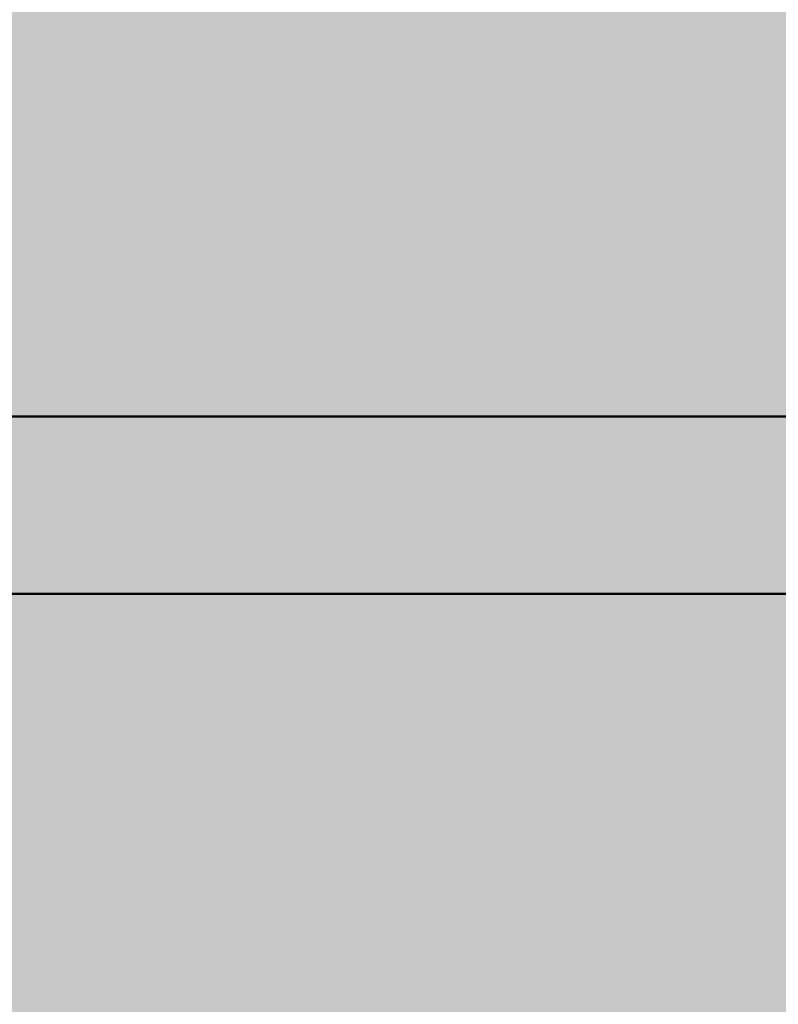
# Model space of a CAD drawing. Units: millimetres. Extents: x 0 to 2267, y 0 to 1823.
# Tile 132 of 256: x 1611 to 1632, y 1216 to 1243. Entities that reach past the tile are written whole.
import ezdxf

# ---------------------------------------------------------------- set-up
doc = ezdxf.new("R2010")
doc.units = ezdxf.units.MM
doc.header["$MEASUREMENT"] = 0
doc.layers.add('M-HATC', color=252, linetype='Continuous', lineweight=18)
doc.layers.add('M-OUTL', color=7, linetype='Continuous', lineweight=50)

msp = doc.modelspace()

# ---------------------------------------------------------------- hatches: boundary and pattern name
at = {"layer": 'M-HATC'}
h = msp.add_hatch(color=256, dxfattribs=at)
h.dxf.hatch_style = 1
h.paths.add_polyline_path([(2065.771, 1618.062, 0.236068), (2055.771, 1638.062), (1381.087, 1638.062, 0.236068), (1371.087, 1618.062), (1371.087, 1603.062), (2055.771, 1603.062), (2065.771, 1603.062)])
h.paths.add_polyline_path([(2062.772, 1550.296), (2062.772, 1560.296), (1374.086, 1560.296), (1374.086, 1550.296), (1374.086, 1540.296), (1384.086, 1540.296), (1389.086, 1540.296), (2062.772, 1540.296)])
h.paths.add_polyline_path([(1930.929, 1282.766), (1505.929, 1282.766), (1587.628, 1235.597, 0.131652), (1600.128, 1232.247), (1836.73, 1232.247, 0.131652), (1849.23, 1235.597)])
h.paths.add_polyline_path([(1930.929, 1117.417), (1905.929, 1117.417), (1505.929, 1117.417), (1505.929, 1077.417), (1930.929, 1077.417)])
h = msp.add_hatch(color=256, dxfattribs=at)
h.dxf.hatch_style = 1
h.paths.add_polyline_path([(2055.771, 1603.062), (1381.087, 1603.062), (1381.087, 1598.062), (2055.771, 1598.062)])
h.paths.add_polyline_path([(2055.771, 1598.062), (1381.087, 1598.062), (1381.087, 1593.062), (2055.771, 1593.062)])
h.paths.add_polyline_path([(2051.307, 1536.761), (1385.55, 1536.761), (1385.55, 1526.761), (1387.55, 1526.761), (1388.537, 1525.053), (1385.332, 1521.233), (1385.332, 1521.223), (2050.254, 1522.749), (2048.321, 1525.053), (2049.307, 1526.761), (2051.307, 1526.761)])
edge = h.paths.add_edge_path()
edge.add_arc((1847.535, 1379.149), 135, 222.60306, 222.89085, ccw=False)
edge.add_line((1748.166, 1287.766), (1683.092, 1287.766))
edge.add_arc((1583.724, 1379.149), 135, 317.10915, 317.39694, ccw=False)
edge.add_arc((1678.969, 1290.671), 5, 222.8909, 317.1091, ccw=False)
edge.add_arc((1774.213, 1379.149), 135, 222.60306, 222.89085, ccw=False)
edge.add_line((1674.845, 1287.766), (1609.771, 1287.766))
edge.add_arc((1510.403, 1379.149), 135, 317.10915, 317.39694, ccw=False)
edge.add_arc((1605.647, 1290.671), 5, 222.8909, 317.1091, ccw=False)
edge.add_arc((1700.892, 1379.149), 135, 222.60306, 222.89085, ccw=False)
edge.add_line((1601.524, 1287.766), (1536.45, 1287.766))
edge.add_arc((1437.081, 1379.149), 135, 317.10915, 317.39694, ccw=False)
edge.add_arc((1532.326, 1290.671), 5, 222.8909, 317.1091, ccw=False)
edge.add_arc((1627.571, 1379.149), 135, 222.60306, 222.89085, ccw=False)
edge.add_line((1528.203, 1287.766), (1505.929, 1287.766))
edge.add_spline(control_points=[(1505.929, 1287.766), (1504.262, 1287.766), (1504.262, 1282.766), (1505.929, 1282.766)], knot_values=[0, 0, 0, 0, 5, 5, 5, 5], degree=3, periodic=0)
edge.add_line((1505.929, 1282.766), (1930.929, 1282.766))
edge.add_spline(control_points=[(1930.929, 1282.766), (1932.596, 1282.766), (1932.596, 1287.766), (1930.929, 1287.766)], knot_values=[0, 0, 0, 0, 5, 5, 5, 5], degree=3, periodic=0)
edge.add_line((1930.929, 1287.766), (1903.056, 1287.766))
edge.add_arc((1803.688, 1379.149), 135, 317.10915, 317.39694, ccw=False)
edge.add_arc((1898.932, 1290.671), 5, 222.8909, 317.1091, ccw=False)
edge.add_arc((1994.177, 1379.149), 135, 222.60306, 222.89085, ccw=False)
edge.add_line((1894.809, 1287.766), (1829.735, 1287.766))
edge.add_arc((1730.366, 1379.149), 135, 317.10915, 317.39694, ccw=False)
edge.add_arc((1825.611, 1290.671), 5, 222.8909, 317.1091, ccw=False)
edge.add_arc((1920.856, 1379.149), 135, 222.60306, 222.89085, ccw=False)
edge.add_line((1821.487, 1287.766), (1756.413, 1287.766))
edge.add_arc((1657.045, 1379.149), 135, 317.10915, 317.39694, ccw=False)
edge.add_arc((1752.29, 1290.671), 5, 222.8909, 317.1091, ccw=False)
edge = h.paths.add_edge_path()
edge.add_spline(control_points=[(1843.429, 1227.247), (1845.096, 1227.247), (1845.096, 1232.247), (1843.429, 1232.247)], knot_values=[0, 0, 0, 0, 5, 5, 5, 5], degree=3, periodic=0)
edge.add_line((1843.429, 1232.247), (1593.429, 1232.247))
edge.add_spline(control_points=[(1593.429, 1232.247), (1591.762, 1232.247), (1591.762, 1227.247), (1593.429, 1227.247)], knot_values=[0, 0, 0, 0, 5, 5, 5, 5], degree=3, periodic=0)
edge.add_line((1593.429, 1227.247), (1843.429, 1227.247))
h.paths.add_polyline_path([(1905.929, 1127.417), (1530.929, 1127.417, 0.414214), (1520.929, 1117.417), (1530.929, 1117.417), (1915.929, 1117.417, 0.414214)])
edge = h.paths.add_edge_path()
edge.add_arc((1397.086, 1498.408), 12.73, 90.7821, 190.8787, ccw=False)
edge.add_line((1396.912, 1511.136), (1428.01, 1511.349))
edge.add_line((1428.01, 1511.349), (1433.01, 1511.349))
edge.add_line((1433.01, 1511.349), (1434.439, 1511.349))
edge.add_arc((1419.474, 1498.08), 20, 41.561, 74.0821)
edge.add_line((1424.959, 1517.314), (1399.935, 1517.256))
edge.add_spline(control_points=[(1399.931, 1517.256), (1399.884, 1517.213), (1399.833, 1517.169), (1399.777, 1517.124)], knot_values=[11.567499, 11.567499, 11.567499, 11.567499, 11.814249, 11.814249, 11.814249, 11.814249], degree=3, periodic=0)
edge.add_spline(control_points=[(1399.633, 1517.01), (1399.583, 1516.972), (1399.531, 1516.934), (1399.476, 1516.895)], knot_values=[11.167718, 11.167718, 11.167718, 11.167718, 11.365188, 11.365188, 11.365188, 11.365188], degree=3, periodic=0)
edge.add_spline(control_points=[(1399.34, 1516.8), (1399.151, 1516.672), (1398.938, 1516.538), (1398.704, 1516.399)], knot_values=[10.376405, 10.376405, 10.376405, 10.376405, 11.00994, 11.00994, 11.00994, 11.00994], degree=3, periodic=0)
edge.add_spline(control_points=[(1398.657, 1516.372), (1398.579, 1516.326), (1398.498, 1516.28), (1398.415, 1516.233)], knot_values=[10.125175, 10.125175, 10.125175, 10.125175, 10.334406, 10.334406, 10.334406, 10.334406], degree=3, periodic=0)
edge.add_spline(control_points=[(1398.264, 1516.149), (1398.196, 1516.111), (1398.126, 1516.073), (1398.055, 1516.035)], knot_values=[9.832246, 9.832246, 9.832246, 9.832246, 9.999658, 9.999658, 9.999658, 9.999658], degree=3, periodic=0)
edge.add_spline(control_points=[(1397.999, 1516.005), (1397.731, 1515.862), (1397.446, 1515.717), (1397.147, 1515.571)], knot_values=[9.161808, 9.161808, 9.161808, 9.161808, 9.787769, 9.787769, 9.787769, 9.787769], degree=3, periodic=0)
edge.add_spline(control_points=[(1397.147, 1515.571), (1396.842, 1515.423), (1396.522, 1515.274), (1396.191, 1515.126)], knot_values=[8.524455, 8.524455, 8.524455, 8.524455, 9.161808, 9.161808, 9.161808, 9.161808], degree=3, periodic=0)
edge.add_spline(control_points=[(1396.078, 1515.076), (1395.985, 1515.035), (1395.892, 1514.994), (1395.798, 1514.953)], knot_values=[8.275193, 8.275193, 8.275193, 8.275193, 8.451726, 8.451726, 8.451726, 8.451726], degree=3, periodic=0)
edge.add_spline(control_points=[(1395.602, 1514.869), (1395.5, 1514.826), (1395.397, 1514.782), (1395.293, 1514.739)], knot_values=[7.962917, 7.962917, 7.962917, 7.962917, 8.152764, 8.152764, 8.152764, 8.152764], degree=3, periodic=0)
edge.add_spline(control_points=[(1395.212, 1514.706), (1394.828, 1514.547), (1394.435, 1514.393), (1394.036, 1514.244)], knot_values=[7.21254, 7.21254, 7.21254, 7.21254, 7.913148, 7.913148, 7.913148, 7.913148], degree=3, periodic=0)
edge.add_spline(control_points=[(1394.036, 1514.244), (1393.708, 1514.121), (1393.375, 1514.003), (1393.043, 1513.889)], knot_values=[6.633733, 6.633733, 6.633733, 6.633733, 7.21254, 7.21254, 7.21254, 7.21254], degree=3, periodic=0)
edge.add_spline(control_points=[(1392.821, 1513.815), (1392.72, 1513.781), (1392.618, 1513.748), (1392.517, 1513.715)], knot_values=[6.328796, 6.328796, 6.328796, 6.328796, 6.505493, 6.505493, 6.505493, 6.505493], degree=3, periodic=0)
edge.add_spline(control_points=[(1392.517, 1513.715), (1392.319, 1513.652), (1392.121, 1513.59), (1391.924, 1513.531)], knot_values=[5.984605, 5.984605, 5.984605, 5.984605, 6.328796, 6.328796, 6.328796, 6.328796], degree=3, periodic=0)
edge.add_spline(control_points=[(1391.792, 1513.491), (1391.312, 1513.35), (1390.838, 1513.224), (1390.378, 1513.117)], knot_values=[5.066697, 5.066697, 5.066697, 5.066697, 5.907055, 5.907055, 5.907055, 5.907055], degree=3, periodic=0)
edge.add_spline(control_points=[(1390.378, 1513.117), (1390.18, 1513.071), (1389.984, 1513.028), (1389.791, 1512.99)], knot_values=[4.70367, 4.70367, 4.70367, 4.70367, 5.066695, 5.066695, 5.066695, 5.066695], degree=3, periodic=0)
edge.add_spline(control_points=[(1389.422, 1512.92), (1389.246, 1512.889), (1389.073, 1512.862), (1388.904, 1512.838)], knot_values=[4.130571, 4.130571, 4.130571, 4.130571, 4.469816, 4.469816, 4.469816, 4.469816], degree=3, periodic=0)
edge.add_spline(control_points=[(1388.904, 1512.838), (1388.591, 1512.795), (1388.291, 1512.764), (1388.007, 1512.749)], knot_values=[3.504031, 3.504031, 3.504031, 3.504031, 4.130571, 4.130571, 4.130571, 4.130571], degree=3, periodic=0)
edge.add_spline(control_points=[(1387.936, 1512.746), (1387.854, 1512.742), (1387.773, 1512.74), (1387.694, 1512.739)], knot_values=[3.268866, 3.268866, 3.268866, 3.268866, 3.451164, 3.451164, 3.451164, 3.451164], degree=3, periodic=0)
edge.add_spline(control_points=[(1387.335, 1512.744), (1387.208, 1512.75), (1387.085, 1512.76), (1386.967, 1512.774)], knot_values=[2.670686, 2.670686, 2.670686, 2.670686, 2.984, 2.984, 2.984, 2.984], degree=3, periodic=0)
edge.add_spline(control_points=[(1386.833, 1512.792), (1386.821, 1512.794), (1386.809, 1512.796), (1386.797, 1512.798)], knot_values=[2.516981, 2.516981, 2.516981, 2.516981, 2.549528, 2.549528, 2.549528, 2.549528], degree=3, periodic=0)
edge.add_spline(control_points=[(1386.453, 1512.873), (1386.426, 1512.881), (1386.399, 1512.889), (1386.373, 1512.897)], knot_values=[2.095869, 2.095869, 2.095869, 2.095869, 2.17941, 2.17941, 2.17941, 2.17941], degree=3, periodic=0)
edge.add_spline(control_points=[(1386.069, 1513.019), (1386.063, 1513.022), (1386.058, 1513.025), (1386.052, 1513.028)], knot_values=[1.72453, 1.72453, 1.72453, 1.72453, 1.745933, 1.745933, 1.745933, 1.745933], degree=3, periodic=0)
edge.add_arc((1399.474, 1498.08), 20, 131.8243, 180)
edge.add_arc((1630.334, 1505.548), 250.971, 181.70518, 236.42798)
edge.add_arc((1605.34, 1483.304), 218.782, 238.66083, 243.34961)
edge.add_arc((1647.091, 1510.359), 262.899, 183.12984, 237.85344, ccw=False)
h.paths.add_polyline_path([(1406.537, 1391.964, 0.149382), (1491.551, 1296.442, -0.129517)], flags=17)
edge = h.paths.add_edge_path()
edge.add_arc((2037.384, 1498.08), 20, 0, 48.2659)
edge.add_spline(control_points=[(2050.697, 1513.005), (2050.651, 1512.985), (2050.603, 1512.966), (2050.554, 1512.948)], knot_values=[1.835652, 1.835652, 1.835652, 1.835652, 2.000781, 2.000781, 2.000781, 2.000781], degree=3, periodic=0)
edge.add_spline(control_points=[(2050.462, 1512.917), (2050.479, 1512.922), (2050.496, 1512.928), (2050.513, 1512.934)], knot_values=[2.045477, 2.045477, 2.045477, 2.045477, 2.101389, 2.101389, 2.101389, 2.101389], degree=3, periodic=0)
edge.add_spline(control_points=[(2050.129, 1512.834), (2050.198, 1512.847), (2050.266, 1512.862), (2050.331, 1512.879)], knot_values=[2.237629, 2.237629, 2.237629, 2.237629, 2.435841, 2.435841, 2.435841, 2.435841], degree=3, periodic=0)
edge.add_spline(control_points=[(2050.095, 1512.828), (2050.106, 1512.83), (2050.118, 1512.832), (2050.129, 1512.834)], knot_values=[2.435841, 2.435841, 2.435841, 2.435841, 2.468321, 2.468321, 2.468321, 2.468321], degree=3, periodic=0)
edge.add_spline(control_points=[(2049.784, 1512.785), (2049.855, 1512.792), (2049.924, 1512.801), (2049.992, 1512.811)], knot_values=[2.563852, 2.563852, 2.563852, 2.563852, 2.748541, 2.748541, 2.748541, 2.748541], degree=3, periodic=0)
edge.add_spline(control_points=[(2049.405, 1512.762), (2049.536, 1512.765), (2049.663, 1512.773), (2049.784, 1512.785)], knot_values=[2.748541, 2.748541, 2.748541, 2.748541, 3.064882, 3.064882, 3.064882, 3.064882], degree=3, periodic=0)
edge.add_spline(control_points=[(2049.17, 1512.76), (2049.234, 1512.759), (2049.297, 1512.759), (2049.358, 1512.761)], knot_values=[3.102309, 3.102309, 3.102309, 3.102309, 3.2503, 3.2503, 3.2503, 3.2503], degree=3, periodic=0)
edge.add_spline(control_points=[(2048.857, 1512.769), (2048.964, 1512.764), (2049.068, 1512.761), (2049.17, 1512.76)], knot_values=[3.2503, 3.2503, 3.2503, 3.2503, 3.486069, 3.486069, 3.486069, 3.486069], degree=3, periodic=0)
edge.add_spline(control_points=[(2048.692, 1512.779), (2048.373, 1512.801), (2048.035, 1512.841), (2047.682, 1512.897)], knot_values=[3.606429, 3.606429, 3.606429, 3.606429, 4.2989, 4.2989, 4.2989, 4.2989], degree=3, periodic=0)
edge.add_spline(control_points=[(2047.682, 1512.897), (2047.546, 1512.919), (2047.408, 1512.942), (2047.268, 1512.969)], knot_values=[4.2989, 4.2989, 4.2989, 4.2989, 4.565769, 4.565769, 4.565769, 4.565769], degree=3, periodic=0)
edge.add_spline(control_points=[(2047.268, 1512.969), (2047.145, 1512.991), (2047.021, 1513.016), (2046.895, 1513.042)], knot_values=[4.565769, 4.565769, 4.565769, 4.565769, 4.799971, 4.799971, 4.799971, 4.799971], degree=3, periodic=0)
edge.add_spline(control_points=[(2046.895, 1513.042), (2046.529, 1513.119), (2046.151, 1513.209), (2045.768, 1513.311)], knot_values=[4.799971, 4.799971, 4.799971, 4.799971, 5.483718, 5.483718, 5.483718, 5.483718], degree=3, periodic=0)
edge.add_spline(control_points=[(2045.768, 1513.311), (2045.372, 1513.415), (2044.97, 1513.532), (2044.566, 1513.659)], knot_values=[5.483718, 5.483718, 5.483718, 5.483718, 6.187866, 6.187866, 6.187866, 6.187866], degree=3, periodic=0)
edge.add_spline(control_points=[(2044.566, 1513.659), (2044.415, 1513.706), (2044.263, 1513.755), (2044.112, 1513.805)], knot_values=[6.187866, 6.187866, 6.187866, 6.187866, 6.451551, 6.451551, 6.451551, 6.451551], degree=3, periodic=0)
edge.add_spline(control_points=[(2044.112, 1513.805), (2043.997, 1513.843), (2043.882, 1513.881), (2043.767, 1513.92)], knot_values=[6.451551, 6.451551, 6.451551, 6.451551, 6.651434, 6.651434, 6.651434, 6.651434], degree=3, periodic=0)
edge.add_spline(control_points=[(2043.767, 1513.92), (2043.372, 1514.055), (2042.977, 1514.198), (2042.589, 1514.346)], knot_values=[6.651434, 6.651434, 6.651434, 6.651434, 7.338879, 7.338879, 7.338879, 7.338879], degree=3, periodic=0)
edge.add_spline(control_points=[(2042.589, 1514.346), (2042.164, 1514.507), (2041.746, 1514.675), (2041.341, 1514.846)], knot_values=[7.338879, 7.338879, 7.338879, 7.338879, 8.089209, 8.089209, 8.089209, 8.089209], degree=3, periodic=0)
edge.add_spline(control_points=[(2041.341, 1514.846), (2041.103, 1514.946), (2040.869, 1515.048), (2040.64, 1515.15)], knot_values=[8.089209, 8.089209, 8.089209, 8.089209, 8.529587, 8.529587, 8.529587, 8.529587], degree=3, periodic=0)
edge.add_spline(control_points=[(2040.51, 1515.209), (2040.082, 1515.402), (2039.675, 1515.597), (2039.295, 1515.789)], knot_values=[8.613818, 8.613818, 8.613818, 8.613818, 9.44571, 9.44571, 9.44571, 9.44571], degree=3, periodic=0)
edge.add_spline(control_points=[(2039.295, 1515.789), (2039.062, 1515.907), (2038.839, 1516.025), (2038.629, 1516.14)], knot_values=[9.44571, 9.44571, 9.44571, 9.44571, 9.956404, 9.956404, 9.956404, 9.956404], degree=3, periodic=0)
edge.add_spline(control_points=[(2038.629, 1516.14), (2038.519, 1516.2), (2038.412, 1516.26), (2038.309, 1516.319)], knot_values=[9.956404, 9.956404, 9.956404, 9.956404, 10.223542, 10.223542, 10.223542, 10.223542], degree=3, periodic=0)
edge.add_spline(control_points=[(2038.309, 1516.319), (2038.214, 1516.374), (2038.122, 1516.428), (2038.033, 1516.481)], knot_values=[10.223542, 10.223542, 10.223542, 10.223542, 10.47051, 10.47051, 10.47051, 10.47051], degree=3, periodic=0)
edge.add_spline(control_points=[(2038.033, 1516.481), (2037.786, 1516.63), (2037.564, 1516.773), (2037.372, 1516.909)], knot_values=[10.47051, 10.47051, 10.47051, 10.47051, 11.15767, 11.15767, 11.15767, 11.15767], degree=3, periodic=0)
edge.add_spline(control_points=[(2037.372, 1516.909), (2037.279, 1516.975), (2037.193, 1517.04), (2037.114, 1517.102)], knot_values=[11.15767, 11.15767, 11.15767, 11.15767, 11.49227, 11.49227, 11.49227, 11.49227], degree=3, periodic=0)
edge.add_spline(control_points=[(2036.856, 1517.326), (2036.915, 1517.269), (2036.981, 1517.21), (2037.056, 1517.149)], knot_values=[11.577341, 11.577341, 11.577341, 11.577341, 11.91035, 11.91035, 11.91035, 11.91035], degree=3, periodic=0)
edge.add_spline(control_points=[(2036.807, 1517.375), (2036.823, 1517.359), (2036.839, 1517.342), (2036.856, 1517.326)], knot_values=[11.91035, 11.91035, 11.91035, 11.91035, 12.007402, 12.007402, 12.007402, 12.007402], degree=3, periodic=0)
edge.add_spline(control_points=[(2036.702, 1517.494), (2036.71, 1517.483), (2036.72, 1517.472), (2036.729, 1517.461)], knot_values=[12.184155, 12.184155, 12.184155, 12.184155, 12.255409, 12.255409, 12.255409, 12.255409], degree=3, periodic=0)
edge.add_spline(control_points=[(2036.616, 1517.621), (2036.62, 1517.613), (2036.624, 1517.606), (2036.629, 1517.598)], knot_values=[12.487913, 12.487913, 12.487913, 12.487913, 12.541035, 12.541035, 12.541035, 12.541035], degree=3, periodic=0)
edge.add_spline(control_points=[(2036.563, 1517.786), (2036.564, 1517.779), (2036.564, 1517.773), (2036.565, 1517.766)], knot_values=[12.911761, 12.911761, 12.911761, 12.911761, 12.968286, 12.968286, 12.968286, 12.968286], degree=3, periodic=0)
edge.add_spline(control_points=[(2036.617, 1517.93), (2036.612, 1517.926), (2036.609, 1517.921), (2036.605, 1517.916)], knot_values=[13.382527, 13.382527, 13.382527, 13.382527, 13.433791, 13.433791, 13.433791, 13.433791], degree=3, periodic=0)
edge.add_spline(control_points=[(2036.749, 1518.017), (2036.736, 1518.012), (2036.724, 1518.006), (2036.712, 1518)], knot_values=[13.726299, 13.726299, 13.726299, 13.726299, 13.809928, 13.809928, 13.809928, 13.809928], degree=3, periodic=0)
edge.add_spline(control_points=[(2036.86, 1518.053), (2036.839, 1518.047), (2036.818, 1518.042), (2036.799, 1518.035)], knot_values=[13.910887, 13.910887, 13.910887, 13.910887, 14.02153, 14.02153, 14.02153, 14.02153], degree=3, periodic=0)
edge.add_line((2036.964, 1518.08), (2032.384, 1518.08))
edge.add_line((2032.384, 1518.08), (2027.384, 1518.08))
edge.add_line((2027.384, 1518.08), (2022.384, 1518.08))
edge.add_line((2022.384, 1518.08), (2017.384, 1518.08))
edge.add_arc((2017.384, 1498.08), 20, 90, 138.439)
edge.add_line((2002.419, 1511.349), (2003.848, 1511.349))
edge.add_line((2003.848, 1511.349), (2008.848, 1511.349))
edge.add_line((2008.848, 1511.349), (2039.772, 1511.138))
edge.add_arc((2039.772, 1498.408), 12.73, -10.8787, 90, ccw=False)
edge.add_arc((1789.767, 1510.359), 262.899, 302.14656, 356.87016, ccw=False)
edge.add_arc((1831.518, 1483.304), 218.782, 296.65039, 301.33917)
edge.add_arc((1806.524, 1505.548), 250.971, 303.57202, 358.29482)
h.paths.add_polyline_path([(2030.321, 1391.964, -0.129517), (1945.307, 1296.442, 0.149382)], flags=17)
edge = h.paths.add_edge_path()
edge.add_spline(control_points=[(2037.246, 1518.082), (2037.29, 1518.081), (2037.336, 1518.08), (2037.384, 1518.08)], knot_values=[0.000012, 0.000012, 0.000012, 0.000012, 0.144754, 0.144754, 0.144754, 0.144754], degree=3, periodic=0)
edge.add_line((2037.336, 1518.08), (2037.01, 1518.08))
edge.add_spline(control_points=[(2037.01, 1518.08), (2036.982, 1518.077), (2036.956, 1518.073), (2036.931, 1518.068)], knot_values=[14.13465, 14.13465, 14.13465, 14.13465, 14.247197, 14.247197, 14.247197, 14.247197], degree=3, periodic=0)
edge.add_spline(control_points=[(2036.931, 1518.068), (2036.928, 1518.067), (2036.924, 1518.067), (2036.921, 1518.066)], knot_values=[14.118315, 14.118315, 14.118315, 14.118315, 14.13465, 14.13465, 14.13465, 14.13465], degree=3, periodic=0)
edge.add_spline(control_points=[(2036.921, 1518.066), (2036.912, 1518.064), (2036.903, 1518.063), (2036.895, 1518.061)], knot_values=[14.078086, 14.078086, 14.078086, 14.078086, 14.118315, 14.118315, 14.118315, 14.118315], degree=3, periodic=0)
edge.add_spline(control_points=[(2036.895, 1518.061), (2036.883, 1518.058), (2036.872, 1518.056), (2036.86, 1518.053)], knot_values=[14.02153, 14.02153, 14.02153, 14.02153, 14.078086, 14.078086, 14.078086, 14.078086], degree=3, periodic=0)
edge.add_spline(control_points=[(2036.86, 1518.053), (2036.839, 1518.047), (2036.818, 1518.042), (2036.799, 1518.035)], knot_values=[13.910887, 13.910887, 13.910887, 13.910887, 14.02153, 14.02153, 14.02153, 14.02153], degree=3, periodic=0)
edge.add_spline(control_points=[(2036.799, 1518.035), (2036.798, 1518.035), (2036.797, 1518.035), (2036.797, 1518.035)], knot_values=[13.906906, 13.906906, 13.906906, 13.906906, 13.910887, 13.910887, 13.910887, 13.910887], degree=3, periodic=0)
edge.add_spline(control_points=[(2036.797, 1518.035), (2036.788, 1518.032), (2036.78, 1518.029), (2036.772, 1518.026)], knot_values=[13.857826, 13.857826, 13.857826, 13.857826, 13.906906, 13.906906, 13.906906, 13.906906], degree=3, periodic=0)
edge.add_spline(control_points=[(2036.772, 1518.026), (2036.764, 1518.023), (2036.756, 1518.02), (2036.749, 1518.017)], knot_values=[13.809928, 13.809928, 13.809928, 13.809928, 13.857826, 13.857826, 13.857826, 13.857826], degree=3, periodic=0)
edge.add_spline(control_points=[(2036.749, 1518.017), (2036.736, 1518.012), (2036.724, 1518.006), (2036.712, 1518)], knot_values=[13.726299, 13.726299, 13.726299, 13.726299, 13.809928, 13.809928, 13.809928, 13.809928], degree=3, periodic=0)
edge.add_spline(control_points=[(2036.712, 1518), (2036.712, 1518), (2036.712, 1518), (2036.711, 1518)], knot_values=[13.723993, 13.723993, 13.723993, 13.723993, 13.726299, 13.726299, 13.726299, 13.726299], degree=3, periodic=0)
edge.add_spline(control_points=[(2036.711, 1518), (2036.706, 1517.997), (2036.701, 1517.994), (2036.696, 1517.992)], knot_values=[13.686536, 13.686536, 13.686536, 13.686536, 13.723993, 13.723993, 13.723993, 13.723993], degree=3, periodic=0)
edge.add_spline(control_points=[(2036.696, 1517.992), (2036.692, 1517.989), (2036.687, 1517.987), (2036.683, 1517.984)], knot_values=[13.651251, 13.651251, 13.651251, 13.651251, 13.686536, 13.686536, 13.686536, 13.686536], degree=3, periodic=0)
edge.add_spline(control_points=[(2036.683, 1517.984), (2036.676, 1517.98), (2036.67, 1517.976), (2036.664, 1517.971)], knot_values=[13.596804, 13.596804, 13.596804, 13.596804, 13.651251, 13.651251, 13.651251, 13.651251], degree=3, periodic=0)
edge.add_spline(control_points=[(2036.664, 1517.971), (2036.664, 1517.971), (2036.663, 1517.971), (2036.663, 1517.971)], knot_values=[13.593956, 13.593956, 13.593956, 13.593956, 13.596804, 13.596804, 13.596804, 13.596804], degree=3, periodic=0)
edge.add_spline(control_points=[(2036.663, 1517.971), (2036.66, 1517.969), (2036.658, 1517.967), (2036.655, 1517.965)], knot_values=[13.570322, 13.570322, 13.570322, 13.570322, 13.593956, 13.593956, 13.593956, 13.593956], degree=3, periodic=0)
edge.add_spline(control_points=[(2036.655, 1517.965), (2036.653, 1517.963), (2036.65, 1517.961), (2036.647, 1517.959)], knot_values=[13.545477, 13.545477, 13.545477, 13.545477, 13.570322, 13.570322, 13.570322, 13.570322], degree=3, periodic=0)
edge.add_spline(control_points=[(2036.647, 1517.959), (2036.647, 1517.959), (2036.647, 1517.959), (2036.647, 1517.959)], knot_values=[13.543931, 13.543931, 13.543931, 13.543931, 13.545477, 13.545477, 13.545477, 13.545477], degree=3, periodic=0)
edge.add_spline(control_points=[(2036.647, 1517.959), (2036.641, 1517.954), (2036.636, 1517.949), (2036.631, 1517.945)], knot_values=[13.488237, 13.488237, 13.488237, 13.488237, 13.543931, 13.543931, 13.543931, 13.543931], degree=3, periodic=0)
edge.add_spline(control_points=[(2036.631, 1517.945), (2036.628, 1517.942), (2036.626, 1517.94), (2036.623, 1517.937)], knot_values=[13.460307, 13.460307, 13.460307, 13.460307, 13.488237, 13.488237, 13.488237, 13.488237], degree=3, periodic=0)
edge.add_spline(control_points=[(2036.623, 1517.937), (2036.622, 1517.936), (2036.62, 1517.934), (2036.618, 1517.932)], knot_values=[13.439712, 13.439712, 13.439712, 13.439712, 13.460307, 13.460307, 13.460307, 13.460307], degree=3, periodic=0)
edge.add_spline(control_points=[(2036.618, 1517.932), (2036.618, 1517.931), (2036.617, 1517.931), (2036.617, 1517.93)], knot_values=[13.433791, 13.433791, 13.433791, 13.433791, 13.439712, 13.439712, 13.439712, 13.439712], degree=3, periodic=0)
edge.add_spline(control_points=[(2036.617, 1517.93), (2036.612, 1517.926), (2036.609, 1517.921), (2036.605, 1517.916)], knot_values=[13.382527, 13.382527, 13.382527, 13.382527, 13.433791, 13.433791, 13.433791, 13.433791], degree=3, periodic=0)
edge.add_spline(control_points=[(2036.605, 1517.916), (2036.603, 1517.913), (2036.6, 1517.91), (2036.598, 1517.907)], knot_values=[13.350017, 13.350017, 13.350017, 13.350017, 13.382527, 13.382527, 13.382527, 13.382527], degree=3, periodic=0)
edge.add_spline(control_points=[(2036.598, 1517.907), (2036.597, 1517.906), (2036.596, 1517.904), (2036.595, 1517.903)], knot_values=[13.333922, 13.333922, 13.333922, 13.333922, 13.350017, 13.350017, 13.350017, 13.350017], degree=3, periodic=0)
edge.add_spline(control_points=[(2036.595, 1517.903), (2036.595, 1517.902), (2036.594, 1517.901), (2036.593, 1517.9)], knot_values=[13.323828, 13.323828, 13.323828, 13.323828, 13.333922, 13.333922, 13.333922, 13.333922], degree=3, periodic=0)
edge.add_spline(control_points=[(2036.593, 1517.9), (2036.59, 1517.895), (2036.588, 1517.891), (2036.585, 1517.886)], knot_values=[13.277545, 13.277545, 13.277545, 13.277545, 13.323828, 13.323828, 13.323828, 13.323828], degree=3, periodic=0)
edge.add_spline(control_points=[(2036.585, 1517.886), (2036.584, 1517.883), (2036.582, 1517.879), (2036.58, 1517.875)], knot_values=[13.240119, 13.240119, 13.240119, 13.240119, 13.277545, 13.277545, 13.277545, 13.277545], degree=3, periodic=0)
edge.add_spline(control_points=[(2036.58, 1517.875), (2036.58, 1517.874), (2036.579, 1517.873), (2036.578, 1517.872)], knot_values=[13.228211, 13.228211, 13.228211, 13.228211, 13.240119, 13.240119, 13.240119, 13.240119], degree=3, periodic=0)
edge.add_spline(control_points=[(2036.578, 1517.872), (2036.578, 1517.87), (2036.577, 1517.869), (2036.577, 1517.868)], knot_values=[13.215717, 13.215717, 13.215717, 13.215717, 13.228211, 13.228211, 13.228211, 13.228211], degree=3, periodic=0)
edge.add_spline(control_points=[(2036.577, 1517.868), (2036.575, 1517.864), (2036.574, 1517.86), (2036.573, 1517.857)], knot_values=[13.179847, 13.179847, 13.179847, 13.179847, 13.215717, 13.215717, 13.215717, 13.215717], degree=3, periodic=0)
edge.add_spline(control_points=[(2036.573, 1517.857), (2036.571, 1517.851), (2036.57, 1517.846), (2036.569, 1517.841)], knot_values=[13.132017, 13.132017, 13.132017, 13.132017, 13.179847, 13.179847, 13.179847, 13.179847], degree=3, periodic=0)
edge.add_spline(control_points=[(2036.569, 1517.841), (2036.568, 1517.84), (2036.568, 1517.839), (2036.568, 1517.838)], knot_values=[13.122482, 13.122482, 13.122482, 13.122482, 13.132017, 13.132017, 13.132017, 13.132017], degree=3, periodic=0)
edge.add_spline(control_points=[(2036.568, 1517.838), (2036.568, 1517.836), (2036.567, 1517.835), (2036.567, 1517.833)], knot_values=[13.105592, 13.105592, 13.105592, 13.105592, 13.122482, 13.122482, 13.122482, 13.122482], degree=3, periodic=0)
edge.add_spline(control_points=[(2036.567, 1517.833), (2036.566, 1517.829), (2036.566, 1517.826), (2036.565, 1517.822)], knot_values=[13.074063, 13.074063, 13.074063, 13.074063, 13.105592, 13.105592, 13.105592, 13.105592], degree=3, periodic=0)
edge.add_spline(control_points=[(2036.565, 1517.822), (2036.565, 1517.822), (2036.565, 1517.822), (2036.565, 1517.822)], knot_values=[13.074043, 13.074043, 13.074043, 13.074043, 13.074063, 13.074063, 13.074063, 13.074063], degree=3, periodic=0)
edge.add_spline(control_points=[(2036.565, 1517.822), (2036.564, 1517.816), (2036.564, 1517.811), (2036.564, 1517.805)], knot_values=[13.021884, 13.021884, 13.021884, 13.021884, 13.074043, 13.074043, 13.074043, 13.074043], degree=3, periodic=0)
edge.add_spline(control_points=[(2036.564, 1517.805), (2036.564, 1517.804), (2036.564, 1517.803), (2036.564, 1517.803)], knot_values=[13.01674, 13.01674, 13.01674, 13.01674, 13.021884, 13.021884, 13.021884, 13.021884], degree=3, periodic=0)
edge.add_spline(control_points=[(2036.564, 1517.803), (2036.563, 1517.801), (2036.563, 1517.798), (2036.563, 1517.796)], knot_values=[12.996438, 12.996438, 12.996438, 12.996438, 13.01674, 13.01674, 13.01674, 13.01674], degree=3, periodic=0)
edge.add_spline(control_points=[(2036.563, 1517.796), (2036.563, 1517.793), (2036.563, 1517.789), (2036.563, 1517.786)], knot_values=[12.968286, 12.968286, 12.968286, 12.968286, 12.996438, 12.996438, 12.996438, 12.996438], degree=3, periodic=0)
edge.add_spline(control_points=[(2036.563, 1517.786), (2036.564, 1517.779), (2036.564, 1517.773), (2036.565, 1517.766)], knot_values=[12.911761, 12.911761, 12.911761, 12.911761, 12.968286, 12.968286, 12.968286, 12.968286], degree=3, periodic=0)
edge.add_spline(control_points=[(2036.565, 1517.766), (2036.565, 1517.766), (2036.565, 1517.766), (2036.565, 1517.766)], knot_values=[12.911017, 12.911017, 12.911017, 12.911017, 12.911761, 12.911761, 12.911761, 12.911761], degree=3, periodic=0)
edge.add_spline(control_points=[(2036.565, 1517.766), (2036.565, 1517.762), (2036.566, 1517.759), (2036.566, 1517.756)], knot_values=[12.88528, 12.88528, 12.88528, 12.88528, 12.911017, 12.911017, 12.911017, 12.911017], degree=3, periodic=0)
edge.add_spline(control_points=[(2036.566, 1517.756), (2036.567, 1517.753), (2036.567, 1517.751), (2036.568, 1517.748)], knot_values=[12.862519, 12.862519, 12.862519, 12.862519, 12.88528, 12.88528, 12.88528, 12.88528], degree=3, periodic=0)
edge.add_spline(control_points=[(2036.568, 1517.748), (2036.568, 1517.747), (2036.568, 1517.747), (2036.568, 1517.746)], knot_values=[12.858885, 12.858885, 12.858885, 12.858885, 12.862519, 12.862519, 12.862519, 12.862519], degree=3, periodic=0)
edge.add_spline(control_points=[(2036.568, 1517.746), (2036.569, 1517.74), (2036.571, 1517.733), (2036.572, 1517.726)], knot_values=[12.8053, 12.8053, 12.8053, 12.8053, 12.858885, 12.858885, 12.858885, 12.858885], degree=3, periodic=0)
edge.add_spline(control_points=[(2036.572, 1517.726), (2036.573, 1517.723), (2036.574, 1517.719), (2036.576, 1517.715)], knot_values=[12.775176, 12.775176, 12.775176, 12.775176, 12.8053, 12.8053, 12.8053, 12.8053], degree=3, periodic=0)
edge.add_spline(control_points=[(2036.576, 1517.715), (2036.576, 1517.713), (2036.577, 1517.71), (2036.578, 1517.708)], knot_values=[12.756759, 12.756759, 12.756759, 12.756759, 12.775176, 12.775176, 12.775176, 12.775176], degree=3, periodic=0)
edge.add_spline(control_points=[(2036.578, 1517.708), (2036.578, 1517.707), (2036.578, 1517.706), (2036.579, 1517.705)], knot_values=[12.748742, 12.748742, 12.748742, 12.748742, 12.756759, 12.756759, 12.756759, 12.756759], degree=3, periodic=0)
edge.add_spline(control_points=[(2036.579, 1517.705), (2036.581, 1517.698), (2036.583, 1517.692), (2036.586, 1517.685)], knot_values=[12.69959, 12.69959, 12.69959, 12.69959, 12.748742, 12.748742, 12.748742, 12.748742], degree=3, periodic=0)
edge.add_spline(control_points=[(2036.586, 1517.685), (2036.588, 1517.68), (2036.59, 1517.675), (2036.592, 1517.669)], knot_values=[12.659038, 12.659038, 12.659038, 12.659038, 12.69959, 12.69959, 12.69959, 12.69959], degree=3, periodic=0)
edge.add_spline(control_points=[(2036.592, 1517.669), (2036.594, 1517.665), (2036.596, 1517.66), (2036.598, 1517.656)], knot_values=[12.626806, 12.626806, 12.626806, 12.626806, 12.659038, 12.659038, 12.659038, 12.659038], degree=3, periodic=0)
edge.add_spline(control_points=[(2036.598, 1517.656), (2036.598, 1517.655), (2036.599, 1517.654), (2036.599, 1517.653)], knot_values=[12.619394, 12.619394, 12.619394, 12.619394, 12.626806, 12.626806, 12.626806, 12.626806], degree=3, periodic=0)
edge.add_spline(control_points=[(2036.599, 1517.653), (2036.604, 1517.642), (2036.61, 1517.632), (2036.616, 1517.621)], knot_values=[12.541039, 12.541039, 12.541039, 12.541039, 12.619394, 12.619394, 12.619394, 12.619394], degree=3, periodic=0)
edge.add_spline(control_points=[(2036.616, 1517.621), (2036.616, 1517.621), (2036.616, 1517.621), (2036.616, 1517.621)], knot_values=[12.541035, 12.541035, 12.541035, 12.541035, 12.541039, 12.541039, 12.541039, 12.541039], degree=3, periodic=0)
edge.add_spline(control_points=[(2036.616, 1517.621), (2036.62, 1517.613), (2036.624, 1517.606), (2036.629, 1517.598)], knot_values=[12.487913, 12.487913, 12.487913, 12.487913, 12.541035, 12.541035, 12.541035, 12.541035], degree=3, periodic=0)
edge.add_spline(control_points=[(2036.629, 1517.598), (2036.633, 1517.592), (2036.637, 1517.585), (2036.641, 1517.579)], knot_values=[12.443982, 12.443982, 12.443982, 12.443982, 12.487913, 12.487913, 12.487913, 12.487913], degree=3, periodic=0)
edge.add_spline(control_points=[(2036.641, 1517.579), (2036.641, 1517.578), (2036.642, 1517.576), (2036.643, 1517.575)], knot_values=[12.434996, 12.434996, 12.434996, 12.434996, 12.443982, 12.443982, 12.443982, 12.443982], degree=3, periodic=0)
edge.add_spline(control_points=[(2036.643, 1517.575), (2036.653, 1517.56), (2036.664, 1517.544), (2036.676, 1517.528)], knot_values=[12.329647, 12.329647, 12.329647, 12.329647, 12.434996, 12.434996, 12.434996, 12.434996], degree=3, periodic=0)
edge.add_spline(control_points=[(2036.676, 1517.528), (2036.684, 1517.517), (2036.693, 1517.505), (2036.702, 1517.494)], knot_values=[12.255409, 12.255409, 12.255409, 12.255409, 12.329647, 12.329647, 12.329647, 12.329647], degree=3, periodic=0)
edge.add_spline(control_points=[(2036.702, 1517.494), (2036.71, 1517.483), (2036.72, 1517.472), (2036.729, 1517.461)], knot_values=[12.184155, 12.184155, 12.184155, 12.184155, 12.255409, 12.255409, 12.255409, 12.255409], degree=3, periodic=0)
edge.add_spline(control_points=[(2036.729, 1517.461), (2036.744, 1517.444), (2036.759, 1517.426), (2036.775, 1517.409)], knot_values=[12.075961, 12.075961, 12.075961, 12.075961, 12.184155, 12.184155, 12.184155, 12.184155], degree=3, periodic=0)
edge.add_spline(control_points=[(2036.775, 1517.409), (2036.776, 1517.407), (2036.777, 1517.406), (2036.778, 1517.405)], knot_values=[12.069502, 12.069502, 12.069502, 12.069502, 12.075961, 12.075961, 12.075961, 12.075961], degree=3, periodic=0)
edge.add_spline(control_points=[(2036.778, 1517.405), (2036.788, 1517.395), (2036.797, 1517.385), (2036.807, 1517.375)], knot_values=[12.007402, 12.007402, 12.007402, 12.007402, 12.069502, 12.069502, 12.069502, 12.069502], degree=3, periodic=0)
edge.add_spline(control_points=[(2036.807, 1517.375), (2036.823, 1517.359), (2036.839, 1517.342), (2036.856, 1517.326)], knot_values=[11.91035, 11.91035, 11.91035, 11.91035, 12.007402, 12.007402, 12.007402, 12.007402], degree=3, periodic=0)
edge.add_spline(control_points=[(2036.856, 1517.326), (2036.915, 1517.269), (2036.981, 1517.21), (2037.056, 1517.149)], knot_values=[11.577341, 11.577341, 11.577341, 11.577341, 11.91035, 11.91035, 11.91035, 11.91035], degree=3, periodic=0)
edge.add_spline(control_points=[(2037.056, 1517.149), (2037.075, 1517.134), (2037.094, 1517.118), (2037.114, 1517.102)], knot_values=[11.49227, 11.49227, 11.49227, 11.49227, 11.577341, 11.577341, 11.577341, 11.577341], degree=3, periodic=0)
edge.add_spline(control_points=[(2037.114, 1517.102), (2037.193, 1517.04), (2037.279, 1516.975), (2037.372, 1516.909)], knot_values=[11.15767, 11.15767, 11.15767, 11.15767, 11.49227, 11.49227, 11.49227, 11.49227], degree=3, periodic=0)
edge.add_spline(control_points=[(2037.372, 1516.909), (2037.564, 1516.773), (2037.786, 1516.63), (2038.033, 1516.481)], knot_values=[10.47051, 10.47051, 10.47051, 10.47051, 11.15767, 11.15767, 11.15767, 11.15767], degree=3, periodic=0)
edge.add_spline(control_points=[(2038.033, 1516.481), (2038.122, 1516.428), (2038.214, 1516.374), (2038.309, 1516.319)], knot_values=[10.223542, 10.223542, 10.223542, 10.223542, 10.47051, 10.47051, 10.47051, 10.47051], degree=3, periodic=0)
edge.add_spline(control_points=[(2038.309, 1516.319), (2038.412, 1516.26), (2038.519, 1516.2), (2038.629, 1516.14)], knot_values=[9.956404, 9.956404, 9.956404, 9.956404, 10.223542, 10.223542, 10.223542, 10.223542], degree=3, periodic=0)
edge.add_spline(control_points=[(2038.629, 1516.14), (2038.839, 1516.025), (2039.062, 1515.907), (2039.295, 1515.789)], knot_values=[9.44571, 9.44571, 9.44571, 9.44571, 9.956404, 9.956404, 9.956404, 9.956404], degree=3, periodic=0)
edge.add_spline(control_points=[(2039.295, 1515.789), (2039.675, 1515.597), (2040.082, 1515.402), (2040.51, 1515.209)], knot_values=[8.613818, 8.613818, 8.613818, 8.613818, 9.44571, 9.44571, 9.44571, 9.44571], degree=3, periodic=0)
edge.add_spline(control_points=[(2040.51, 1515.209), (2040.553, 1515.189), (2040.597, 1515.17), (2040.64, 1515.15)], knot_values=[8.529587, 8.529587, 8.529587, 8.529587, 8.613818, 8.613818, 8.613818, 8.613818], degree=3, periodic=0)
edge.add_spline(control_points=[(2040.64, 1515.15), (2040.869, 1515.048), (2041.103, 1514.946), (2041.341, 1514.846)], knot_values=[8.089209, 8.089209, 8.089209, 8.089209, 8.529587, 8.529587, 8.529587, 8.529587], degree=3, periodic=0)
edge.add_spline(control_points=[(2041.341, 1514.846), (2041.746, 1514.675), (2042.164, 1514.507), (2042.589, 1514.346)], knot_values=[7.338879, 7.338879, 7.338879, 7.338879, 8.089209, 8.089209, 8.089209, 8.089209], degree=3, periodic=0)
edge.add_spline(control_points=[(2042.589, 1514.346), (2042.977, 1514.198), (2043.372, 1514.055), (2043.767, 1513.92)], knot_values=[6.651434, 6.651434, 6.651434, 6.651434, 7.338879, 7.338879, 7.338879, 7.338879], degree=3, periodic=0)
edge.add_spline(control_points=[(2043.767, 1513.92), (2043.882, 1513.881), (2043.997, 1513.843), (2044.112, 1513.805)], knot_values=[6.451551, 6.451551, 6.451551, 6.451551, 6.651434, 6.651434, 6.651434, 6.651434], degree=3, periodic=0)
edge.add_spline(control_points=[(2044.112, 1513.805), (2044.263, 1513.755), (2044.415, 1513.706), (2044.566, 1513.659)], knot_values=[6.187866, 6.187866, 6.187866, 6.187866, 6.451551, 6.451551, 6.451551, 6.451551], degree=3, periodic=0)
edge.add_spline(control_points=[(2044.566, 1513.659), (2044.97, 1513.532), (2045.372, 1513.415), (2045.768, 1513.311)], knot_values=[5.483718, 5.483718, 5.483718, 5.483718, 6.187866, 6.187866, 6.187866, 6.187866], degree=3, periodic=0)
edge.add_spline(control_points=[(2045.768, 1513.311), (2046.151, 1513.209), (2046.529, 1513.119), (2046.895, 1513.042)], knot_values=[4.799971, 4.799971, 4.799971, 4.799971, 5.483718, 5.483718, 5.483718, 5.483718], degree=3, periodic=0)
edge.add_spline(control_points=[(2046.895, 1513.042), (2047.021, 1513.016), (2047.145, 1512.991), (2047.268, 1512.969)], knot_values=[4.565769, 4.565769, 4.565769, 4.565769, 4.799971, 4.799971, 4.799971, 4.799971], degree=3, periodic=0)
edge.add_spline(control_points=[(2047.268, 1512.969), (2047.408, 1512.942), (2047.546, 1512.919), (2047.682, 1512.897)], knot_values=[4.2989, 4.2989, 4.2989, 4.2989, 4.565769, 4.565769, 4.565769, 4.565769], degree=3, periodic=0)
edge.add_spline(control_points=[(2047.682, 1512.897), (2048.035, 1512.841), (2048.373, 1512.801), (2048.692, 1512.779)], knot_values=[3.606429, 3.606429, 3.606429, 3.606429, 4.2989, 4.2989, 4.2989, 4.2989], degree=3, periodic=0)
edge.add_spline(control_points=[(2048.692, 1512.779), (2048.748, 1512.775), (2048.803, 1512.772), (2048.857, 1512.769)], knot_values=[3.486069, 3.486069, 3.486069, 3.486069, 3.606429, 3.606429, 3.606429, 3.606429], degree=3, periodic=0)
edge.add_spline(control_points=[(2048.857, 1512.769), (2048.964, 1512.764), (2049.068, 1512.761), (2049.17, 1512.76)], knot_values=[3.2503, 3.2503, 3.2503, 3.2503, 3.486069, 3.486069, 3.486069, 3.486069], degree=3, periodic=0)
edge.add_spline(control_points=[(2049.17, 1512.76), (2049.234, 1512.759), (2049.297, 1512.759), (2049.358, 1512.761)], knot_values=[3.102309, 3.102309, 3.102309, 3.102309, 3.2503, 3.2503, 3.2503, 3.2503], degree=3, periodic=0)
edge.add_spline(control_points=[(2049.358, 1512.761), (2049.374, 1512.761), (2049.39, 1512.761), (2049.405, 1512.762)], knot_values=[3.064882, 3.064882, 3.064882, 3.064882, 3.102309, 3.102309, 3.102309, 3.102309], degree=3, periodic=0)
edge.add_spline(control_points=[(2049.405, 1512.762), (2049.536, 1512.765), (2049.663, 1512.773), (2049.784, 1512.785)], knot_values=[2.748541, 2.748541, 2.748541, 2.748541, 3.064882, 3.064882, 3.064882, 3.064882], degree=3, periodic=0)
edge.add_spline(control_points=[(2049.784, 1512.785), (2049.855, 1512.792), (2049.924, 1512.801), (2049.992, 1512.811)], knot_values=[2.563852, 2.563852, 2.563852, 2.563852, 2.748541, 2.748541, 2.748541, 2.748541], degree=3, periodic=0)
edge.add_spline(control_points=[(2049.992, 1512.811), (2050.026, 1512.816), (2050.061, 1512.822), (2050.095, 1512.828)], knot_values=[2.468321, 2.468321, 2.468321, 2.468321, 2.563852, 2.563852, 2.563852, 2.563852], degree=3, periodic=0)
edge.add_spline(control_points=[(2050.095, 1512.828), (2050.106, 1512.83), (2050.118, 1512.832), (2050.129, 1512.834)], knot_values=[2.435841, 2.435841, 2.435841, 2.435841, 2.468321, 2.468321, 2.468321, 2.468321], degree=3, periodic=0)
edge.add_spline(control_points=[(2050.129, 1512.834), (2050.198, 1512.847), (2050.266, 1512.862), (2050.331, 1512.879)], knot_values=[2.237629, 2.237629, 2.237629, 2.237629, 2.435841, 2.435841, 2.435841, 2.435841], degree=3, periodic=0)
edge.add_spline(control_points=[(2050.331, 1512.879), (2050.375, 1512.891), (2050.419, 1512.903), (2050.462, 1512.917)], knot_values=[2.101389, 2.101389, 2.101389, 2.101389, 2.237629, 2.237629, 2.237629, 2.237629], degree=3, periodic=0)
edge.add_spline(control_points=[(2050.462, 1512.917), (2050.479, 1512.922), (2050.496, 1512.928), (2050.513, 1512.934)], knot_values=[2.045477, 2.045477, 2.045477, 2.045477, 2.101389, 2.101389, 2.101389, 2.101389], degree=3, periodic=0)
edge.add_spline(control_points=[(2050.513, 1512.934), (2050.527, 1512.938), (2050.54, 1512.943), (2050.554, 1512.948)], knot_values=[2.000781, 2.000781, 2.000781, 2.000781, 2.045477, 2.045477, 2.045477, 2.045477], degree=3, periodic=0)
edge.add_spline(control_points=[(2050.554, 1512.948), (2050.603, 1512.966), (2050.651, 1512.985), (2050.697, 1513.005)], knot_values=[1.835652, 1.835652, 1.835652, 1.835652, 2.000781, 2.000781, 2.000781, 2.000781], degree=3, periodic=0)
edge.add_arc((2037.384, 1498.08), 20, 48.2659, 90.1299)
edge = h.paths.add_edge_path(flags=16)
edge.add_spline(control_points=[(1386.139, 1512.986), (1388.92, 1511.739), (1398.039, 1515.519), (1399.931, 1517.256)], knot_values=[1.831046, 1.831046, 1.831046, 1.831046, 11.814249, 11.814249, 11.814249, 11.814249], degree=3, periodic=0)
edge.add_line((1399.931, 1517.256), (1393.743, 1517.242))
edge.add_arc((1399.474, 1498.08), 20, 106.6501, 131.8173)
h = msp.add_hatch(color=256, dxfattribs=at)
h.dxf.hatch_style = 1
h.paths.add_polyline_path([(2042.889, 1580.18), (2055.771, 1593.062), (1381.087, 1593.062), (1393.969, 1580.18), (1374.086, 1560.296), (2062.772, 1560.296)])
h.paths.add_polyline_path([(1843.429, 1201.33), (1843.429, 1227.247), (1593.429, 1227.247), (1593.429, 1201.33, -0.228274), (1574.599, 1162.235), (1530.929, 1127.417), (1905.929, 1127.417), (1862.259, 1162.235, -0.228274)])

# ---------------------------------------------------------------- linework, layer by layer
at = {"layer": 'M-OUTL'}
for p, q in [((1593.429, 1232.247), (1843.429, 1232.247)), ((1593.429, 1227.247), (1843.429, 1227.247))]:
    msp.add_line(p, q, dxfattribs=at)

doc.saveas('drawing.dxf')
